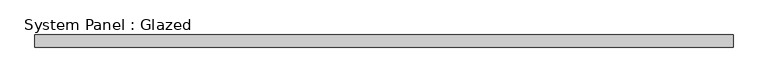
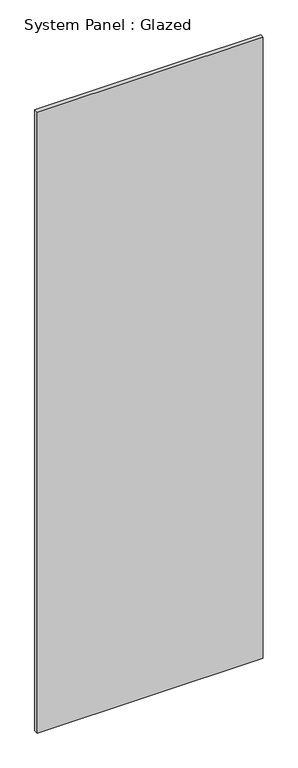
"""IFC4 building model written with IfcOpenShell, lengths in millimetres: plate geometry, System Panel : Glazed."""

from ifc_helpers import new_model, si_unit, origin, origin_with_axes, place, context, project, spatial, polyline, outline, extrude, source, transform, mapped, element, save


def system_panel_glazed_963389ce(model_context):
    return source(origin(), model_context, "Body", "SweptSolid", [
        extrude(outline(polyline([(713.2338716, 19.05), (-713.2338716, 19.05), (-713.2338716, 44.45), (713.2338716, 44.45), (713.2338716, 19.05)])), origin_with_axes(), (0.0, 0.0, 1.0), 4140.2),
    ])


if __name__ == "__main__":
    model = new_model("IFC4")
    model_context = context("Model", 3, world=origin())
    ifc_project = project(units=[si_unit("LENGTHUNIT", "METRE", prefix="MILLI")], contexts=[model_context])
    site = spatial("IfcSite", under=ifc_project)
    building = spatial("IfcBuilding", under=site)
    placement = place(None, origin())
    system_panel_glazed_shape = system_panel_glazed_963389ce(model_context)
    element("IfcPlate", 1, ObjectType="System Panel : Glazed", at=placement, inside=building, context=model_context, shape_type="MappedRepresentation", body=[
        mapped(system_panel_glazed_shape, transform((0.0, 0.0, 0.0), x_axis=(1.0, 0.0, 0.0), y_axis=(0.0, 1.0, 0.0), z_axis=(0.0, 0.0, 1.0))),
    ])
    save(model, "model.ifc")

# Revit data of these elements
# Type "System Panel : Glazed"
#   Construction Type Id = "GSP4R"
#   Analytic Construction = "1/8 in Pilkington single glazing"
#   Visual Light Transmittance = 0.9
#   Solar Heat Gain Coefficient = 0.86
#   Heat Transfer Coefficient (U) = 1.18115 BTU/(h·ft²·°F)
# Element 1 (IfcPlate, "System Panel : Glazed")
#   Materials on its faces: "Glass"
# Materials
#   "Glass": class "Glass", colour RGB 0 128 192, transparency 0.75, Description = "Soda Lime Glass", Cost = 0
